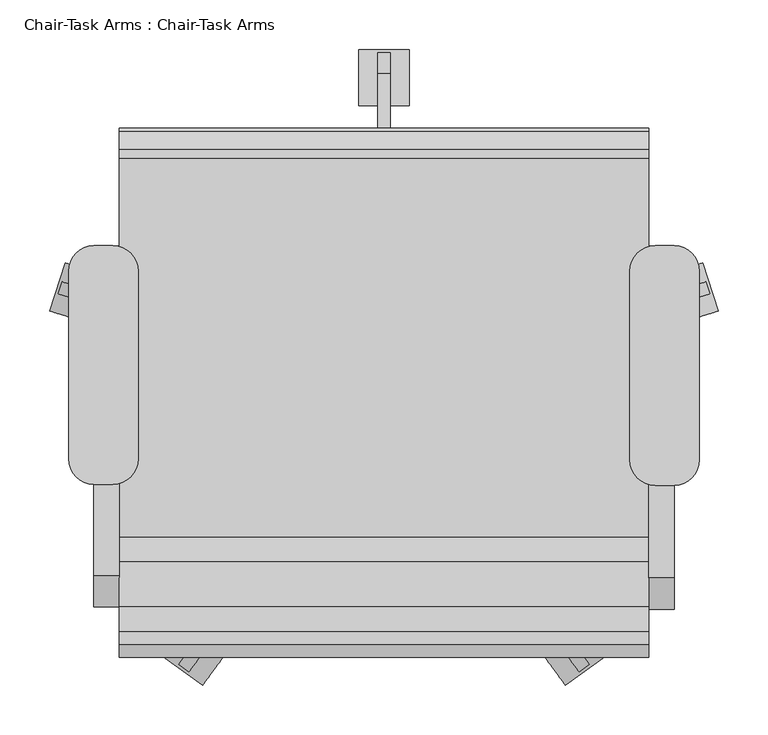
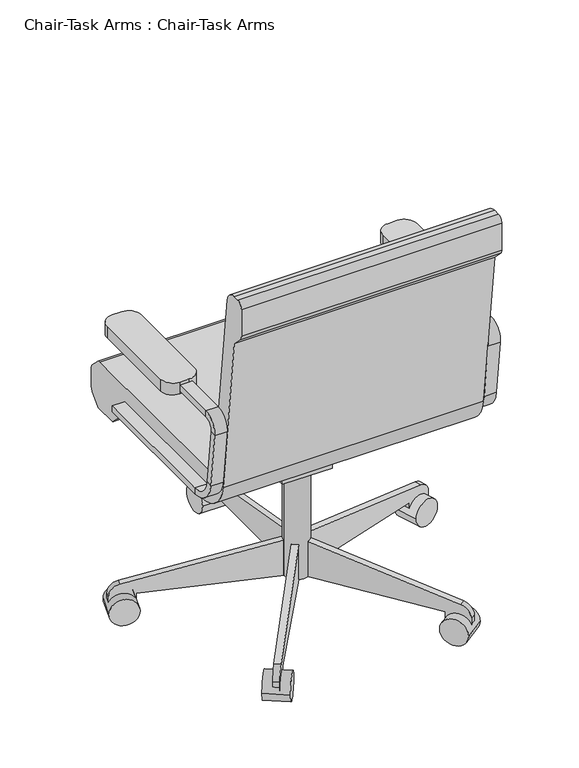
"""IFC4 building model written with IfcOpenShell, lengths in millimetres: furniture geometry, Chair-Task Arms : Chair-Task Arms."""

from ifc_helpers import new_model, si_unit, point, frame, frame_2d, origin, place, context, project, spatial, polyline, circle_curve, trimmed, segment, composite_curve, outline, extrude, source, transform, mapped, element, save
from ifc_brep_helpers import plane_surface, cylinder_surface, revolved_surface, advanced_brep


def chair_task_arms_chair_task_arms_fa5a08ef(model_context):
    return source(origin(), model_context, "Body", "SolidModel", [
        extrude(outline(composite_curve([segment(polyline([(433.0908197, -74.2028048), (414.0408197, -74.2028048)]), True, "CONTINUOUS"), segment(trimmed(circle_curve(frame_2d((414.0408197, -48.8028048)), 25.4), [point((414.0408197, -74.2028048))], [point((388.6408197, -48.8028048))], False, "CARTESIAN"), True, "CONTINUOUS"), segment(polyline([(388.6408197, -48.8028048), (388.6408197, 141.6319091)]), True, "CONTINUOUS"), segment(trimmed(circle_curve(frame_2d((414.0408197, 141.6319091)), 25.4), [point((388.6408197, 141.6319091))], [point((414.0408197, 167.0319091))], False, "CARTESIAN"), True, "CONTINUOUS"), segment(polyline([(414.0408197, 167.0319091), (433.0908197, 167.0319091)]), True, "CONTINUOUS"), segment(trimmed(circle_curve(frame_2d((433.0908197, 141.6319091)), 25.4), [point((433.0908197, 167.0319091))], [point((458.4908197, 141.6319091))], False, "CARTESIAN"), True, "CONTINUOUS"), segment(polyline([(458.4908197, 141.6319091), (458.4908197, -48.8028048)]), True, "CONTINUOUS"), segment(trimmed(circle_curve(frame_2d((433.0908197, -48.8028048)), 25.4), [point((458.4908197, -48.8028048))], [point((433.0908197, -74.2028048))], False, "CARTESIAN"), True, "CONTINUOUS")], self_intersect=False)), frame((0.0, 0.0, 596.9), z_axis=(0.0, 0.0, 1.0), x_axis=(1.0, 0.0, 0.0)), (0.0, 0.0, 1.0), 25.4),
        extrude(outline(composite_curve([segment(polyline([(-132.0591803, -73.1575984), (-151.1091803, -73.1575984)]), True, "CONTINUOUS"), segment(trimmed(circle_curve(frame_2d((-151.1091803, -47.7575984)), 25.4), [point((-151.1091803, -73.1575984))], [point((-176.5091803, -47.7575984))], False, "CARTESIAN"), True, "CONTINUOUS"), segment(polyline([(-176.5091803, -47.7575984), (-176.5091803, 141.6319091)]), True, "CONTINUOUS"), segment(trimmed(circle_curve(frame_2d((-151.1091803, 141.6319091)), 25.4), [point((-176.5091803, 141.6319091))], [point((-151.1091803, 167.0319091))], False, "CARTESIAN"), True, "CONTINUOUS"), segment(polyline([(-151.1091803, 167.0319091), (-132.0591803, 167.0319091)]), True, "CONTINUOUS"), segment(trimmed(circle_curve(frame_2d((-132.0591803, 141.6319091)), 25.4), [point((-132.0591803, 167.0319091))], [point((-106.6591803, 141.6319091))], False, "CARTESIAN"), True, "CONTINUOUS"), segment(polyline([(-106.6591803, 141.6319091), (-106.6591803, -47.7575984)]), True, "CONTINUOUS"), segment(trimmed(circle_curve(frame_2d((-132.0591803, -47.7575984)), 25.4), [point((-106.6591803, -47.7575984))], [point((-132.0591803, -73.1575984))], False, "CARTESIAN"), True, "CONTINUOUS")], self_intersect=False)), frame((0.0, 0.0, 596.9), z_axis=(0.0, 0.0, 1.0), x_axis=(1.0, 0.0, 0.0)), (0.0, 0.0, 1.0), 25.4),
        advanced_brep(
        [(-151.1091803, 167.0319091, 412.75), (-151.1091803, 167.0319091, 425.45), (-125.7091803, 167.0319091, 425.45), (-125.7091803, 167.0319091, 412.75), (-151.1091803, -126.2388651, 412.75), (-151.1091803, -126.2388651, 425.45), (-125.7091803, -126.2388651, 425.45), (-125.7091803, -126.2388651, 412.75), (-151.1091803, -170.3844094, 464.7064065), (-151.1091803, -182.9974221, 463.2225227), (-125.7091803, -170.3844094, 464.7064065), (-125.7091803, -182.9974221, 463.2225227), (-151.1091803, -196.7936301, 580.4902904), (-151.1091803, -184.1806174, 581.9741742), (-125.7091803, -184.1806174, 581.9741742), (-125.7091803, -196.7936301, 580.4902904), (-151.1091803, -165.2610984, 603.25), (-151.1091803, -165.2610984, 615.95), (-125.7091803, -165.2610984, 603.25), (-125.7091803, -165.2610984, 615.95), (-151.1091803, 18.9459016, 615.95), (-125.7091803, 18.9459016, 615.95), (-125.7091803, 18.9459016, 603.25), (-151.1091803, 18.9459016, 603.25)],
        [
            (0, 1),
            (1, 2),
            (2, 3),
            (3, 0),
            (0, 4),
            (4, 5),
            (5, 1),
            (5, 6),
            (6, 2),
            (6, 7),
            (7, 3),
            (7, 4),
            (8, 5, circle_curve(frame((-151.1091803, -126.2388651, 469.9), z_axis=(1.0, 0.0, 0.0), x_axis=(0.0, 0.0, -1.0)), 44.45)),
            (4, 9, circle_curve(frame((-151.1091803, -126.2388651, 469.9), z_axis=(-1.0, 0.0, 0.0), x_axis=(0.0, 0.0, -1.0)), 57.15)),
            (9, 8),
            (10, 6, circle_curve(frame((-125.7091803, -126.2388651, 469.9), z_axis=(1.0, 0.0, 0.0), x_axis=(0.0, 0.0, -1.0)), 44.45)),
            (8, 10),
            (11, 7, circle_curve(frame((-125.7091803, -126.2388651, 469.9), z_axis=(1.0, 0.0, 0.0), x_axis=(0.0, 0.0, -1.0)), 57.15)),
            (10, 11),
            (11, 9),
            (9, 12),
            (12, 13),
            (13, 8),
            (13, 14),
            (14, 10),
            (14, 15),
            (15, 11),
            (15, 12),
            (16, 13, circle_curve(frame((-151.1091803, -165.2610984, 584.2), z_axis=(1.0, 0.0, 0.0), x_axis=(0.0, -0.9931506043228768, -0.11684124756739202)), 19.05)),
            (12, 17, circle_curve(frame((-151.1091803, -165.2610984, 584.2), z_axis=(-1.0, 0.0, 0.0), x_axis=(0.0, -0.9931506043228768, -0.11684124756739202)), 31.75)),
            (17, 16),
            (18, 14, circle_curve(frame((-125.7091803, -165.2610984, 584.2), z_axis=(1.0, 0.0, 0.0), x_axis=(0.0, -0.9931506043228768, -0.11684124756739202)), 19.05)),
            (16, 18),
            (19, 15, circle_curve(frame((-125.7091803, -165.2610984, 584.2), z_axis=(1.0, 0.0, 0.0), x_axis=(0.0, -0.9931506043228768, -0.11684124756739202)), 31.75)),
            (18, 19),
            (19, 17),
            (20, 21),
            (21, 22),
            (22, 23),
            (23, 20),
            (17, 20),
            (23, 16),
            (22, 18),
            (21, 19),
        ],
        [
            plane_surface(frame((-152.608212, 167.0319091, 419.1), z_axis=(0.0, 1.0, 0.0), x_axis=(0.0, 0.0, -1.0))),
            plane_surface(frame((-151.1091803, 167.0319091, 412.75), z_axis=(-1.0, 0.0, 0.0), x_axis=(0.0, -1.0, 0.0))),
            plane_surface(frame((-151.1091803, 167.0319091, 425.45), z_axis=(0.0, 0.0, 1.0), x_axis=(0.0, -1.0, 0.0))),
            plane_surface(frame((-125.7091803, 167.0319091, 425.45), z_axis=(1.0, 0.0, 0.0), x_axis=(0.0, -1.0, 0.0))),
            plane_surface(frame((-125.7091803, 167.0319091, 412.75), z_axis=(0.0, 0.0, -1.0), x_axis=(0.0, -1.0, 0.0))),
            plane_surface(frame((-151.1091803, -126.2388651, 469.9), z_axis=(-1.0, 0.0, 0.0), x_axis=(0.0, 0.0, -1.0))),
            revolved_surface(polyline([(-151.1091803, -126.2388651, 425.45), (-125.7091803, -126.2388651, 425.45)]), (-138.4091803, -126.2388651, 469.9), (-1.0, 0.0, 0.0)),
            plane_surface(frame((-125.7091803, -126.2388651, 469.9), z_axis=(1.0, 0.0, 0.0), x_axis=(0.0, 0.0, -1.0))),
            cylinder_surface(frame((-138.4091803, -126.2388651, 469.9), z_axis=(-1.0, 0.0, 0.0), x_axis=(0.0, 0.0, -1.0)), 57.15),
            plane_surface(frame((-151.1091803, -182.9974221, 463.2225227), z_axis=(-1.0, 0.0, 0.0), x_axis=(0.0, -0.1168412475673856, 0.9931506043228776))),
            plane_surface(frame((-151.1091803, -170.3844094, 464.7064065), z_axis=(0.0, 0.9931506043228776, 0.1168412475673856), x_axis=(0.0, -0.1168412475673856, 0.9931506043228776))),
            plane_surface(frame((-125.7091803, -170.3844094, 464.7064065), z_axis=(1.0, 0.0, 0.0), x_axis=(0.0, -0.1168412475673856, 0.9931506043228776))),
            plane_surface(frame((-125.7091803, -182.9974221, 463.2225227), z_axis=(0.0, -0.9931506043228776, -0.1168412475673856), x_axis=(0.0, -0.1168412475673856, 0.9931506043228776))),
            plane_surface(frame((-151.1091803, -165.2610984, 584.2), z_axis=(-1.0, 0.0, 0.0), x_axis=(0.0, -0.9931506043228768, -0.11684124756739202))),
            revolved_surface(polyline([(-151.1091803, -184.1806174123508, 581.9741742338413), (-125.7091803, -184.1806174123508, 581.9741742338413)]), (-138.4091803, -165.2610984, 584.2), (-1.0, 0.0, 0.0)),
            plane_surface(frame((-125.7091803, -165.2610984, 584.2), z_axis=(1.0, 0.0, 0.0), x_axis=(0.0, -0.9931506043228768, -0.11684124756739202))),
            cylinder_surface(frame((-138.4091803, -165.2610984, 584.2), z_axis=(-1.0, 0.0, 0.0), x_axis=(0.0, -0.9931506043228768, -0.11684124756739202)), 31.75),
            plane_surface(frame((-152.608212, 18.9459016, 609.6), z_axis=(0.0, 1.0, 0.0), x_axis=(0.0, 0.0, 1.0))),
            plane_surface(frame((-151.1091803, -165.2610984, 615.95), z_axis=(-1.0, 0.0, 0.0), x_axis=(0.0, 1.0, 0.0))),
            plane_surface(frame((-151.1091803, -165.2610984, 603.25), z_axis=(0.0, 0.0, -1.0), x_axis=(0.0, 1.0, 0.0))),
            plane_surface(frame((-125.7091803, -165.2610984, 603.25), z_axis=(1.0, 0.0, 0.0), x_axis=(0.0, 1.0, 0.0))),
            plane_surface(frame((-125.7091803, -165.2610984, 615.95), z_axis=(0.0, 0.0, 1.0), x_axis=(0.0, 1.0, 0.0))),
        ],
        [
            (0, [[1, 2, 3, 4]]),
            (1, [[-1, 5, 6, 7]]),
            (2, [[-2, -7, 8, 9]]),
            (3, [[-3, -9, 10, 11]]),
            (4, [[-4, -11, 12, -5]]),
            (5, [[13, -6, 14, 15]]),
            (6, [[16, -8, -13, 17]]),
            (7, [[18, -10, -16, 19]]),
            (8, [[-14, -12, -18, 20]]),
            (9, [[-15, 21, 22, 23]]),
            (10, [[-17, -23, 24, 25]]),
            (11, [[-19, -25, 26, 27]]),
            (12, [[-20, -27, 28, -21]]),
            (13, [[29, -22, 30, 31]]),
            (14, [[32, -24, -29, 33]]),
            (15, [[34, -26, -32, 35]]),
            (16, [[-30, -28, -34, 36]]),
            (17, [[37, 38, 39, 40]]),
            (18, [[-31, 41, -40, 42]]),
            (19, [[-33, -42, -39, 43]]),
            (20, [[-35, -43, -38, 44]]),
            (21, [[-36, -44, -37, -41]]),
        ],
    ),
        advanced_brep(
        [(433.0908197, 167.0319091, 425.45), (433.0908197, 167.0319091, 412.75), (407.6908197, 167.0319091, 412.75), (407.6908197, 167.0319091, 425.45), (433.0908197, -128.329278, 425.45), (433.0908197, -128.329278, 412.75), (407.6908197, -128.329278, 412.75), (407.6908197, -128.329278, 425.45), (433.0908197, -185.0878351, 463.2225227), (433.0908197, -172.4748224, 464.7064065), (407.6908197, -185.0878351, 463.2225227), (407.6908197, -172.4748224, 464.7064065), (433.0908197, -186.2710303, 581.9741742), (433.0908197, -198.884043, 580.4902904), (407.6908197, -198.884043, 580.4902904), (407.6908197, -186.2710303, 581.9741742), (433.0908197, -167.3515113, 615.95), (433.0908197, -167.3515113, 603.25), (407.6908197, -167.3515113, 615.95), (407.6908197, -167.3515113, 603.25), (433.0908197, 18.9459016, 603.25), (407.6908197, 18.9459016, 603.25), (407.6908197, 18.9459016, 615.95), (433.0908197, 18.9459016, 615.95)],
        [
            (0, 1),
            (1, 2),
            (2, 3),
            (3, 0),
            (0, 4),
            (4, 5),
            (5, 1),
            (5, 6),
            (6, 2),
            (6, 7),
            (7, 3),
            (7, 4),
            (8, 5, circle_curve(frame((433.0908197, -128.329278, 469.9), z_axis=(1.0, 0.0, 0.0), x_axis=(0.0, 0.0, -1.0)), 57.15)),
            (4, 9, circle_curve(frame((433.0908197, -128.329278, 469.9), z_axis=(-1.0, 0.0, 0.0), x_axis=(0.0, 0.0, -1.0)), 44.45)),
            (9, 8),
            (10, 6, circle_curve(frame((407.6908197, -128.329278, 469.9), z_axis=(1.0, 0.0, 0.0), x_axis=(0.0, 0.0, -1.0)), 57.15)),
            (8, 10),
            (11, 7, circle_curve(frame((407.6908197, -128.329278, 469.9), z_axis=(1.0, 0.0, 0.0), x_axis=(0.0, 0.0, -1.0)), 44.45)),
            (10, 11),
            (11, 9),
            (9, 12),
            (12, 13),
            (13, 8),
            (13, 14),
            (14, 10),
            (14, 15),
            (15, 11),
            (15, 12),
            (16, 13, circle_curve(frame((433.0908197, -167.3515113, 584.2), z_axis=(1.0, 0.0, 0.0), x_axis=(0.0, -0.9931506043228767, -0.1168412475673929)), 31.75)),
            (12, 17, circle_curve(frame((433.0908197, -167.3515113, 584.2), z_axis=(-1.0, 0.0, 0.0), x_axis=(0.0, -0.9931506043228767, -0.1168412475673929)), 19.05)),
            (17, 16),
            (18, 14, circle_curve(frame((407.6908197, -167.3515113, 584.2), z_axis=(1.0, 0.0, 0.0), x_axis=(0.0, -0.9931506043228767, -0.1168412475673929)), 31.75)),
            (16, 18),
            (19, 15, circle_curve(frame((407.6908197, -167.3515113, 584.2), z_axis=(1.0, 0.0, 0.0), x_axis=(0.0, -0.9931506043228767, -0.1168412475673929)), 19.05)),
            (18, 19),
            (19, 17),
            (20, 21),
            (21, 22),
            (22, 23),
            (23, 20),
            (17, 20),
            (23, 16),
            (22, 18),
            (21, 19),
        ],
        [
            plane_surface(frame((406.191788, 167.0319091, 419.1), z_axis=(0.0, 1.0, 0.0), x_axis=(0.0, 0.0, -1.0))),
            plane_surface(frame((433.0908197, 167.0319091, 425.45), z_axis=(1.0, 0.0, 0.0), x_axis=(0.0, -1.0, 0.0))),
            plane_surface(frame((433.0908197, 167.0319091, 412.75), z_axis=(0.0, 0.0, -1.0), x_axis=(0.0, -1.0, 0.0))),
            plane_surface(frame((407.6908197, 167.0319091, 412.75), z_axis=(-1.0, 0.0, 0.0), x_axis=(0.0, -1.0, 0.0))),
            plane_surface(frame((407.6908197, 167.0319091, 425.45), z_axis=(0.0, 0.0, 1.0), x_axis=(0.0, -1.0, 0.0))),
            plane_surface(frame((433.0908197, -128.329278, 469.9), z_axis=(1.0, 0.0, 0.0), x_axis=(0.0, 0.0, -1.0))),
            cylinder_surface(frame((420.3908197, -128.329278, 469.9), z_axis=(-1.0, 0.0, 0.0), x_axis=(0.0, 0.0, -1.0)), 57.15),
            plane_surface(frame((407.6908197, -128.329278, 469.9), z_axis=(-1.0, 0.0, 0.0), x_axis=(0.0, 0.0, -1.0))),
            revolved_surface(polyline([(407.6908197, -128.329278, 425.45), (433.0908197, -128.329278, 425.45)]), (420.3908197, -128.329278, 469.9), (-1.0, 0.0, 0.0)),
            plane_surface(frame((433.0908197, -172.4748224, 464.7064065), z_axis=(1.0, 0.0, 0.0), x_axis=(0.0, -0.11684124756738626, 0.9931506043228775))),
            plane_surface(frame((433.0908197, -185.0878351, 463.2225227), z_axis=(0.0, -0.9931506043228775, -0.11684124756738655), x_axis=(0.0, -0.11684124756738655, 0.9931506043228775))),
            plane_surface(frame((407.6908197, -185.0878351, 463.2225227), z_axis=(-1.0, 0.0, 0.0), x_axis=(0.0, -0.11684124756738626, 0.9931506043228775))),
            plane_surface(frame((407.6908197, -172.4748224, 464.7064065), z_axis=(0.0, 0.9931506043228775, 0.11684124756738626), x_axis=(0.0, -0.11684124756738626, 0.9931506043228775))),
            plane_surface(frame((433.0908197, -167.3515113, 584.2), z_axis=(1.0, 0.0, 0.0), x_axis=(0.0, -0.9931506043228767, -0.1168412475673929))),
            cylinder_surface(frame((420.3908197, -167.3515113, 584.2), z_axis=(-1.0, 0.0, 0.0), x_axis=(0.0, -0.9931506043228767, -0.1168412475673929)), 31.75),
            plane_surface(frame((407.6908197, -167.3515113, 584.2), z_axis=(-1.0, 0.0, 0.0), x_axis=(0.0, -0.9931506043228767, -0.1168412475673929))),
            revolved_surface(polyline([(407.6908197, -186.2710303123508, 581.9741742338412), (433.0908197, -186.2710303123508, 581.9741742338412)]), (420.3908197, -167.3515113, 584.2), (-1.0, 0.0, 0.0)),
            plane_surface(frame((406.191788, 18.9459016, 609.6), z_axis=(0.0, 1.0, 0.0), x_axis=(0.0, 0.0, 1.0))),
            plane_surface(frame((433.0908197, -167.3515113, 603.25), z_axis=(1.0, 0.0, 0.0), x_axis=(0.0, 1.0, 0.0))),
            plane_surface(frame((433.0908197, -167.3515113, 615.95), z_axis=(0.0, 0.0, 1.0), x_axis=(0.0, 1.0, 0.0))),
            plane_surface(frame((407.6908197, -167.3515113, 615.95), z_axis=(-1.0, 0.0, 0.0), x_axis=(0.0, 1.0, 0.0))),
            plane_surface(frame((407.6908197, -167.3515113, 603.25), z_axis=(0.0, 0.0, -1.0), x_axis=(0.0, 1.0, 0.0))),
        ],
        [
            (0, [[1, 2, 3, 4]]),
            (1, [[-1, 5, 6, 7]]),
            (2, [[-2, -7, 8, 9]]),
            (3, [[-3, -9, 10, 11]]),
            (4, [[-4, -11, 12, -5]]),
            (5, [[13, -6, 14, 15]]),
            (6, [[16, -8, -13, 17]]),
            (7, [[18, -10, -16, 19]]),
            (8, [[-14, -12, -18, 20]]),
            (9, [[-15, 21, 22, 23]]),
            (10, [[-17, -23, 24, 25]]),
            (11, [[-19, -25, 26, 27]]),
            (12, [[-20, -27, 28, -21]]),
            (13, [[29, -22, 30, 31]]),
            (14, [[32, -24, -29, 33]]),
            (15, [[34, -26, -32, 35]]),
            (16, [[-30, -28, -34, 36]]),
            (17, [[37, 38, 39, 40]]),
            (18, [[-31, 41, -40, 42]]),
            (19, [[-33, -42, -39, 43]]),
            (20, [[-35, -43, -38, 44]]),
            (21, [[-36, -44, -37, -41]]),
        ],
    ),
        extrude(outline(composite_curve([segment(trimmed(circle_curve(frame_2d((140.9908197, 18.9459016)), 25.4), [point((115.5908197, 18.9459016))], [point((166.3908197, 18.9459016))], False, "CARTESIAN"), True, "CONTINUOUS"), segment(trimmed(circle_curve(frame_2d((140.9908197, 18.9459016)), 25.4), [point((166.3908197, 18.9459016))], [point((115.5908197, 18.9459016))], False, "CARTESIAN"), True, "CONTINUOUS")], self_intersect=False)), frame((0.0, 0.0, 53.5835944), z_axis=(0.0, 0.0, 1.0), x_axis=(1.0, 0.0, 0.0)), (0.0, 0.0, 1.0), 330.5914056),
        extrude(outline(composite_curve([segment(trimmed(circle_curve(frame_2d((0.0, -28.2002727)), 28.2002727), [point((0.0, -56.4005455))], [point((0.0, 0.0))], False, "CARTESIAN"), True, "CONTINUOUS"), segment(trimmed(circle_curve(frame_2d((0.0, -28.2002727)), 28.2002727), [point((0.0, 0.0))], [point((0.0, -56.4005455))], False, "CARTESIAN"), True, "CONTINUOUS")], self_intersect=False)), frame((477.6203484, 101.6163254, 28.1835944), z_axis=(-0.3090169943749423, 0.9510565162951553, 0.0), x_axis=(0.0, 0.0, 1.0)), (0.0, 0.0, 1.0), 50.8),
        extrude(outline(composite_curve([segment(polyline([(-25.4, 0.0), (0.0, 0.0), (0.0, -50.8), (-24.303053, -50.8)]), True, "CONTINUOUS"), segment(trimmed(circle_curve(frame_2d((-24.303053, -25.4)), 25.4), [point((-24.303053, -50.8))], [point((-49.3171699, -29.8106637))], False, "CARTESIAN"), True, "CONTINUOUS"), segment(polyline([(-49.3171699, -29.8106637), (-101.6, 266.7), (-101.6, 292.1), (-25.4, 292.1), (-25.4, 0.0)]), True, "CONTINUOUS")], self_intersect=False)), frame((420.756686, 103.1705568, 28.1835944), z_axis=(-0.3090169943749423, 0.9510565162951553, 0.0), x_axis=(0.0, 0.0, -1.0)), (0.0, 0.0, 1.0), 12.7),
        extrude(outline(composite_curve([segment(trimmed(circle_curve(frame_2d((0.0, -28.2002727)), 28.2002727), [point((0.0, -56.4005455))], [point((0.0, 0.0))], False, "CARTESIAN"), True, "CONTINUOUS"), segment(trimmed(circle_curve(frame_2d((0.0, -28.2002727)), 28.2002727), [point((0.0, 0.0))], [point((0.0, -56.4005455))], False, "CARTESIAN"), True, "CONTINUOUS")], self_intersect=False)), frame((323.63931, -275.6612394, 28.1835944), z_axis=(0.8090169943749499, 0.5877852522924699, 0.0), x_axis=(0.0, 0.0, 1.0)), (0.0, 0.0, 1.0), 50.8),
        extrude(outline(composite_curve([segment(polyline([(-25.4, 0.0), (0.0, 0.0), (0.0, -50.8), (-24.303053, -50.8)]), True, "CONTINUOUS"), segment(trimmed(circle_curve(frame_2d((-24.303053, -25.3999999)), 25.4), [point((-24.303053, -50.8))], [point((-49.3171699, -29.8106636))], False, "CARTESIAN"), True, "CONTINUOUS"), segment(polyline([(-49.3171699, -29.8106636), (-101.6, 266.7), (-101.6, 292.1), (-25.4, 292.1), (-25.4, 0.0)]), True, "CONTINUOUS")], self_intersect=False)), frame((307.545634, -221.1003988, 28.1835944), z_axis=(0.8090169943749499, 0.5877852522924699, 0.0), x_axis=(0.0, 0.0, -1.0)), (0.0, 0.0, 1.0), 12.7),
        extrude(outline(composite_curve([segment(trimmed(circle_curve(frame_2d((0.0, -28.2002727)), 28.2002727), [point((0.0, -56.4005455))], [point((0.0, 0.0))], False, "CARTESIAN"), True, "CONTINUOUS"), segment(trimmed(circle_curve(frame_2d((0.0, -28.2002727)), 28.2002727), [point((0.0, 0.0))], [point((0.0, -56.4005455))], False, "CARTESIAN"), True, "CONTINUOUS")], self_intersect=False)), frame((-41.6576707, -275.6612394, 28.1835944), z_axis=(-0.8090169943749458, 0.5877852522924754, 0.0), x_axis=(0.0, 0.0, -1.0)), (0.0, 0.0, 1.0), 50.8),
        extrude(outline(composite_curve([segment(polyline([(25.4, 0.0), (25.4, 292.1), (101.6, 292.1), (101.6, 266.7), (49.3171699, -29.8106637)]), True, "CONTINUOUS"), segment(trimmed(circle_curve(frame_2d((24.303053, -25.3999999)), 25.4), [point((49.3171699, -29.8106637))], [point((24.303053, -50.8))], False, "CARTESIAN"), True, "CONTINUOUS"), segment(polyline([(24.303053, -50.8), (0.0, -50.8), (0.0, 0.0), (25.4, 0.0)]), True, "CONTINUOUS")], self_intersect=False)), frame((-25.5639946, -221.1003988, 28.1835944), z_axis=(-0.8090169943749459, 0.5877852522924754, 0.0), x_axis=(0.0, 0.0, 1.0)), (0.0, 0.0, 1.0), 12.7),
        extrude(outline(composite_curve([segment(trimmed(circle_curve(frame_2d((0.0, -28.2002727)), 28.2002727), [point((0.0, -56.4005454))], [point((0.0, 0.0))], False, "CARTESIAN"), True, "CONTINUOUS"), segment(trimmed(circle_curve(frame_2d((0.0, -28.2002727)), 28.2002727), [point((0.0, 0.0))], [point((0.0, -56.4005454))], False, "CARTESIAN"), True, "CONTINUOUS")], self_intersect=False)), frame((-195.638709, 101.6163254, 28.1835944), z_axis=(0.3090169943749487, 0.9510565162951532, 0.0), x_axis=(0.0, 0.0, -1.0)), (0.0, 0.0, 1.0), 50.8),
        extrude(outline(composite_curve([segment(polyline([(25.4, 0.0), (25.4, 292.1000001), (101.6, 292.1000001), (101.6, 266.7), (49.3171699, -29.8106636)]), True, "CONTINUOUS"), segment(trimmed(circle_curve(frame_2d((24.303053, -25.4)), 25.4), [point((49.3171699, -29.8106636))], [point((24.303053, -50.8))], False, "CARTESIAN"), True, "CONTINUOUS"), segment(polyline([(24.303053, -50.8), (0.0, -50.8), (0.0, 0.0), (25.4, 0.0)]), True, "CONTINUOUS")], self_intersect=False)), frame((-138.7750467, 103.1705568, 28.1835944), z_axis=(0.3090169943749487, 0.9510565162951532, 0.0), x_axis=(0.0, 0.0, 1.0)), (0.0, 0.0, 1.0), 12.7),
        extrude(outline(composite_curve([segment(trimmed(circle_curve(frame_2d((336.4459016, 28.1835944)), 28.2002727), [point((308.2456289, 28.1835944))], [point((364.6461744, 28.1835944))], False, "CARTESIAN"), True, "CONTINUOUS"), segment(trimmed(circle_curve(frame_2d((336.4459016, 28.1835944)), 28.2002727), [point((364.6461744, 28.1835944))], [point((308.2456289, 28.1835944))], False, "CARTESIAN"), True, "CONTINUOUS")], self_intersect=False)), frame((115.5908197, 0.0, 0.0), z_axis=(1.0, 0.0, 0.0), x_axis=(0.0, 1.0, 0.0)), (0.0, 0.0, 1.0), 50.8),
        extrude(outline(composite_curve([segment(polyline([(311.0459016, 53.5835944), (18.9459016, 53.5835944), (18.9459016, 129.7835944), (44.3459016, 129.7835944), (340.8565654, 77.5007643)]), True, "CONTINUOUS"), segment(trimmed(circle_curve(frame_2d((336.4459016, 52.4866474)), 25.4), [point((340.8565654, 77.5007643))], [point((361.8459016, 52.4866474))], False, "CARTESIAN"), True, "CONTINUOUS"), segment(polyline([(361.8459016, 52.4866474), (361.8459016, 28.1835944), (311.0459016, 28.1835944), (311.0459016, 53.5835944)]), True, "CONTINUOUS")], self_intersect=False)), frame((134.6408197, 0.0, 0.0), z_axis=(1.0, 0.0, 0.0), x_axis=(0.0, 1.0, 0.0)), (0.0, 0.0, 1.0), 12.7),
        extrude(outline(polyline([(69.7459016, 383.7835944), (69.7459016, 371.0835944), (18.9459016, 283.0954134), (-19.1540984, 283.0954134), (-19.1540984, 383.7835944), (69.7459016, 383.7835944)])), frame((90.1908197, 0.0, 0.0), z_axis=(1.0, 0.0, 0.0), x_axis=(0.0, 1.0, 0.0)), (0.0, 0.0, 1.0), 101.6),
        extrude(outline(composite_curve([segment(polyline([(-126.2050455, 457.2), (255.0102301, 457.2)]), True, "CONTINUOUS"), segment(trimmed(circle_curve(frame_2d((255.0102301, 444.5)), 12.7), [point((255.0102301, 457.2))], [point((263.9604301, 453.510212))], False, "CARTESIAN"), True, "CONTINUOUS"), segment(polyline([(263.9604301, 453.510212), (281.8961016, 435.6939999)]), True, "CONTINUOUS"), segment(trimmed(circle_curve(frame_2d((272.9459016, 426.6837879)), 12.7), [point((281.8961016, 435.6939999))], [point((285.6459016, 426.6837879))], False, "CARTESIAN"), True, "CONTINUOUS"), segment(polyline([(285.6459016, 426.6837879), (285.6459016, 391.6405184)]), True, "CONTINUOUS"), segment(trimmed(circle_curve(frame_2d((260.2459016, 391.6405184)), 25.4), [point((285.6459016, 391.6405184))], [point((278.2663256, 373.7401184))], False, "CARTESIAN"), True, "CONTINUOUS"), segment(polyline([(278.2663256, 373.7401184), (260.2470284, 355.6), (209.4470284, 355.6), (181.0744602, 383.7835944), (-107.1089978, 383.7835944)]), True, "CONTINUOUS"), segment(trimmed(circle_curve(frame_2d((-107.1089978, 459.9835944)), 76.2), [point((-107.1089978, 383.7835944))], [point((-182.7870738, 451.0802913))], False, "CARTESIAN"), True, "CONTINUOUS"), segment(polyline([(-182.7870738, 451.0802913), (-222.3540984, 787.4), (-244.0343545, 809.0802561)]), True, "CONTINUOUS"), segment(trimmed(circle_curve(frame_2d((-235.0540984, 818.0605122)), 12.7), [point((-244.0343545, 809.0802561))], [point((-247.7540984, 818.0605122))], False, "CARTESIAN"), True, "CONTINUOUS"), segment(polyline([(-247.7540984, 818.0605122), (-247.7540984, 876.3)]), True, "CONTINUOUS"), segment(trimmed(circle_curve(frame_2d((-235.0540984, 876.3)), 12.7), [point((-247.7540984, 876.3))], [point((-235.0540984, 889.0))], False, "CARTESIAN"), True, "CONTINUOUS"), segment(polyline([(-235.0540984, 889.0), (-222.1789239, 889.0)]), True, "CONTINUOUS"), segment(trimmed(circle_curve(frame_2d((-222.1789239, 863.6)), 25.4), [point((-222.1789239, 889.0))], [point((-196.9528985, 866.5677677))], False, "CARTESIAN"), True, "CONTINUOUS"), segment(polyline([(-196.9528985, 866.5677677), (-151.4310708, 479.6322323)]), True, "CONTINUOUS"), segment(trimmed(circle_curve(frame_2d((-126.2050455, 482.6)), 25.4), [point((-151.4310708, 479.6322323))], [point((-126.2050455, 457.2))], True, "CARTESIAN"), True, "CONTINUOUS")], self_intersect=False)), frame((-125.7091803, 0.0, 0.0), z_axis=(1.0, 0.0, 0.0), x_axis=(0.0, 1.0, 0.0)), (0.0, 0.0, 1.0), 533.4),
    ])


if __name__ == "__main__":
    model = new_model("IFC4")
    model_context = context("Model", 3, world=origin())
    ifc_project = project(units=[si_unit("LENGTHUNIT", "METRE", prefix="MILLI")], contexts=[model_context])
    site = spatial("IfcSite", under=ifc_project)
    building = spatial("IfcBuilding", under=site)
    placement = place(None, origin())
    chair_task_arms_chair_task_arms_shape = chair_task_arms_chair_task_arms_fa5a08ef(model_context)
    element("IfcFurniture", 1, ObjectType="Chair-Task Arms : Chair-Task Arms", at=placement, inside=building, context=model_context, shape_type="MappedRepresentation", body=[
        mapped(chair_task_arms_chair_task_arms_shape, transform((0.0, 0.0, 0.0), x_axis=(1.0, 0.0, 0.0), y_axis=(0.0, 1.0, 0.0), z_axis=(0.0, 0.0, 1.0))),
    ])
    save(model, "model.ifc")

# Revit data of these elements
# Type "Chair-Task Arms : Chair-Task Arms"
#   Assembly Code = "E2020200"
#   Base Material = Plastic - Black
#   Caster Material = Plastic - Black
#   Seat/Back Material = Textile - Slate Blue
#   Default Elevation = 0
# Element 1 (IfcFurniture, "Chair-Task Arms : Chair-Task Arms")
#   Materials on its faces: "Plastic - Black", "Textile - Slate Blue"
# Materials
#   "Plastic - Black": colour RGB 0 0 0, transparency 0.7
#   "Textile - Slate Blue": colour RGB 98 102 118, transparency 0
